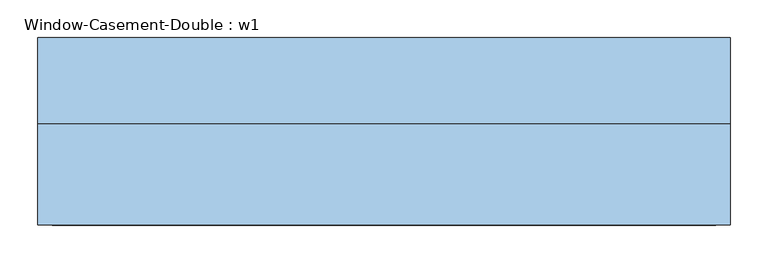
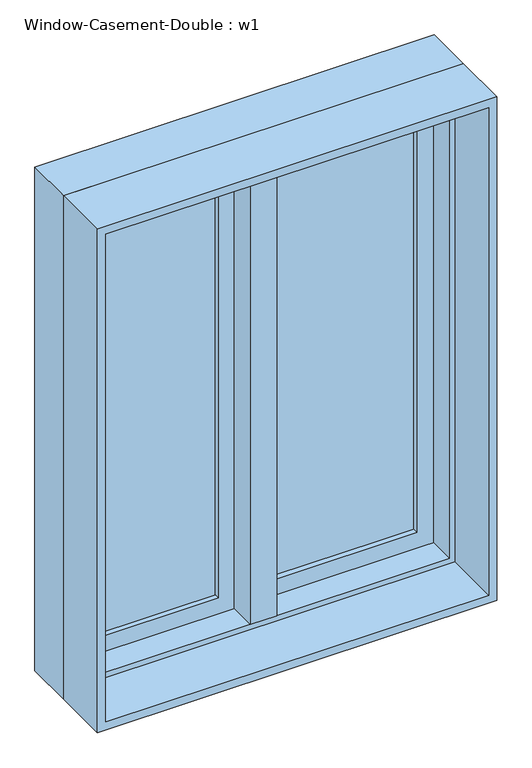
"""IFC4 building model written with IfcOpenShell, lengths in millimetres: window geometry, Window-Casement-Double : w1."""

from ifc_helpers import new_model, si_unit, frame, origin, place, context, project, spatial, polyline, outline, extrude, faceted_brep, source, transform, mapped, element, save


def window_casement_double_w1_d341e8ac(model_context):
    return source(origin(), model_context, "Body", "SolidModel", [
        faceted_brep([(9.525, 133.35, 2120.9), (-9.525, 133.35, 2120.9), (-9.525, 82.55, 2120.9), (9.525, 82.55, 2120.9), (9.525, 133.35, 927.1), (9.525, 82.55, 927.1), (-9.525, 82.55, 927.1), (-9.525, 133.35, 927.1), (-9.525, 82.55, 946.15), (-9.525, 82.55, 2101.85), (-30.1625, 82.55, 946.15), (-30.1625, 82.55, 2101.85), (-30.1625, 19.05, 946.15), (-30.1625, 19.05, 2101.85), (30.1625, 19.05, 946.15), (30.1625, 19.05, 2101.85), (30.1625, 82.55, 946.15), (30.1625, 82.55, 2101.85), (9.525, 82.55, 946.15), (9.525, 82.55, 2101.85)], [[[0, 1, 2, 3]], [[4, 5, 6, 7]], [[1, 0, 4, 7]], [[2, 1, 7, 6, 8, 9]], [[9, 8, 10, 11]], [[11, 10, 12, 13]], [[13, 12, 14, 15]], [[15, 14, 16, 17]], [[17, 16, 18, 19]], [[0, 3, 19, 18, 5, 4]], [[18, 8, 6, 5]], [[9, 19, 3, 2]], [[8, 18, 16, 14, 12, 10]], [[19, 9, 11, 13, 15, 17]]]),
        extrude(outline(polyline([(-66.675, 114.3), (-66.675, 107.95), (-387.35, 107.95), (-387.35, 114.3), (-66.675, 114.3)])), frame((0.0, 0.0, 984.25), z_axis=(0.0, 0.0, 1.0), x_axis=(1.0, 0.0, 0.0)), (0.0, 0.0, 1.0), 1079.5),
        extrude(outline(polyline([(-387.35, 95.25), (-387.35, 101.6), (-66.675, 101.6), (-66.675, 95.25), (-387.35, 95.25)])), frame((0.0, 0.0, 984.25), z_axis=(0.0, 0.0, 1.0), x_axis=(1.0, 0.0, 0.0)), (0.0, 0.0, 1.0), 1079.5),
        extrude(outline(polyline([(387.35, 114.3), (387.35, 107.95), (66.675, 107.95), (66.675, 114.3), (387.35, 114.3)])), frame((0.0, 0.0, 984.25), z_axis=(0.0, 0.0, 1.0), x_axis=(1.0, 0.0, 0.0)), (0.0, 0.0, 1.0), 1079.5),
        extrude(outline(polyline([(66.675, 95.25), (66.675, 101.6), (387.35, 101.6), (387.35, 95.25), (66.675, 95.25)])), frame((0.0, 0.0, 984.25), z_axis=(0.0, 0.0, 1.0), x_axis=(1.0, 0.0, 0.0)), (0.0, 0.0, 1.0), 1079.5),
        extrude(outline(polyline([(2120.9, -444.5), (927.1, -444.5), (927.1, -9.525), (2120.9, -9.525), (2120.9, -444.5)]), holes=[polyline([(2063.75, -66.675), (984.25, -66.675), (984.25, -387.35), (2063.75, -387.35), (2063.75, -66.675)])]), frame((0.0, 82.55, 0.0), z_axis=(0.0, 1.0, 0.0), x_axis=(0.0, 0.0, 1.0)), (0.0, 0.0, 1.0), 44.45),
        extrude(outline(polyline([(927.1, 444.5), (2120.9, 444.5), (2120.9, 9.525), (927.1, 9.525), (927.1, 444.5)]), holes=[polyline([(984.25, 66.675), (2063.75, 66.675), (2063.75, 387.35), (984.25, 387.35), (984.25, 66.675)])]), frame((0.0, 82.55, 0.0), z_axis=(0.0, 1.0, 0.0), x_axis=(0.0, 0.0, 1.0)), (0.0, 0.0, 1.0), 44.45),
        extrude(outline(polyline([(2133.6, -457.2), (914.4, -457.2), (914.4, 457.2), (2133.6, 457.2), (2133.6, -457.2)]), holes=[polyline([(2114.55, 438.15), (933.45, 438.15), (933.45, -438.15), (2114.55, -438.15), (2114.55, 438.15)])]), frame((0.0, -114.3, 0.0), z_axis=(0.0, 1.0, 0.0), x_axis=(0.0, 0.0, 1.0)), (0.0, 0.0, 1.0), 133.35),
        faceted_brep([(425.45, 82.55, 2101.85), (425.45, 19.05, 2101.85), (-425.45, 19.05, 2101.85), (-425.45, 82.55, 2101.85), (444.5, 133.35, 2120.9), (444.5, 82.55, 2120.9), (-444.5, 82.55, 2120.9), (-444.5, 133.35, 2120.9), (457.2, 19.05, 2133.6), (457.2, 133.35, 2133.6), (-457.2, 133.35, 2133.6), (-457.2, 19.05, 2133.6), (-425.45, 19.05, 946.15), (-425.45, 82.55, 946.15), (-444.5, 82.55, 927.1), (-444.5, 133.35, 927.1), (-457.2, 133.35, 914.4), (-457.2, 19.05, 914.4), (425.45, 19.05, 946.15), (425.45, 82.55, 946.15), (444.5, 82.55, 927.1), (444.5, 133.35, 927.1), (457.2, 133.35, 914.4), (457.2, 19.05, 914.4)], [[[0, 1, 2, 3]], [[4, 5, 6, 7]], [[8, 9, 10, 11]], [[3, 2, 12, 13]], [[7, 6, 14, 15]], [[11, 10, 16, 17]], [[13, 12, 18, 19]], [[15, 14, 20, 21]], [[17, 16, 22, 23]], [[11, 17, 23, 8], [1, 18, 12, 2]], [[19, 18, 1, 0]], [[5, 20, 14, 6], [3, 13, 19, 0]], [[21, 20, 5, 4]], [[23, 22, 9, 8]], [[9, 22, 16, 10], [7, 15, 21, 4]]]),
    ])


if __name__ == "__main__":
    model = new_model("IFC4")
    model_context = context("Model", 3, world=origin())
    ifc_project = project(units=[si_unit("LENGTHUNIT", "METRE", prefix="MILLI")], contexts=[model_context])
    site = spatial("IfcSite", under=ifc_project)
    building = spatial("IfcBuilding", under=site)
    placement = place(None, origin())
    window_casement_double_w1_shape = window_casement_double_w1_d341e8ac(model_context)
    element("IfcWindow", 1, ObjectType="Window-Casement-Double : w1", at=placement, inside=building, context=model_context, shape_type="MappedRepresentation", body=[
        mapped(window_casement_double_w1_shape, transform((0.0, 0.0, 0.0), x_axis=(1.0, 0.0, 0.0), y_axis=(0.0, 1.0, 0.0), z_axis=(0.0, 0.0, 1.0))),
    ])
    save(model, "model.ifc")

# Revit data of these elements
# Type "Window-Casement-Double : w1"
#   Type Mark = "14"
#   Fire Rating = "0.5h"
#   Assembly Code = "B2020100"
#   Analytic Construction = "Double glazing - domestic"
#   Frame Extension [instance default] = 0' - 0 1/4"
#   Window Inset [instance default] = 0' - 0"
#   Wall Thickness [instance default] = 0' - 6"
#   Interior Wall Closure [instance default] = 0' - 2 1/4"
#   Half Width = 1' - 6"
#   Visual Light Transmittance = 0.81
#   Thermal Resistance (R) = 1.8146 (h·ft²·°F)/BTU
#   Solar Heat Gain Coefficient = 0.76
#   Rough Width = 3' - 0 1/2"
#   Rough Height = 4' - 0 1/2"
#   Height = 4' - 0"
#   Heat Transfer Coefficient (U) = 0.5511 BTU/(h·ft²·°F)
#   Exterior Wall Closure [instance default] = 0' - 1 1/4"
#   Extension Jamb [instance default] = 0' - 2 1/4"
#   Default Sill Height = 3' - 0"
#   Width = 3' - 0"
#   Define Thermal Properties by = 0
#   Muntin Visibility = yes
#   Interior Trim Visibility [instance default] = yes
#   Exterior Trim Visibility [instance default] = yes
#   Extension Jamb Visibility [instance default] = yes
#   Muntin Pattern = Muntin Pattern_2x2 : Muntin Pattern_2x2
#   Interior Trim = Trim-Window-Interior-Flat : Picture Frame
#   Interior Frame Material = Wood - Stained
#   Glass Panel Material = Glass
#   Exterior Trim = Trim-Window-Exterior-Flat : with Sill
#   Wall Closure = (empty or 0)
# Element 1 (IfcWindow, "Window-Casement-Double : w1")
#   Wall Thickness = 0' - 9"
#   Extension Jamb = 0' - 5 1/4"
#   Materials on its faces: "Wood - Stained", "Glass"
# Materials
#   "Wood - Stained": class "Wood", colour RGB 224 178 126, transparency 0, Cost = 0
#   "Glass": class "Glass", colour RGB 0 128 192, transparency 0.75, Description = "Soda Lime Glass", Cost = 0
